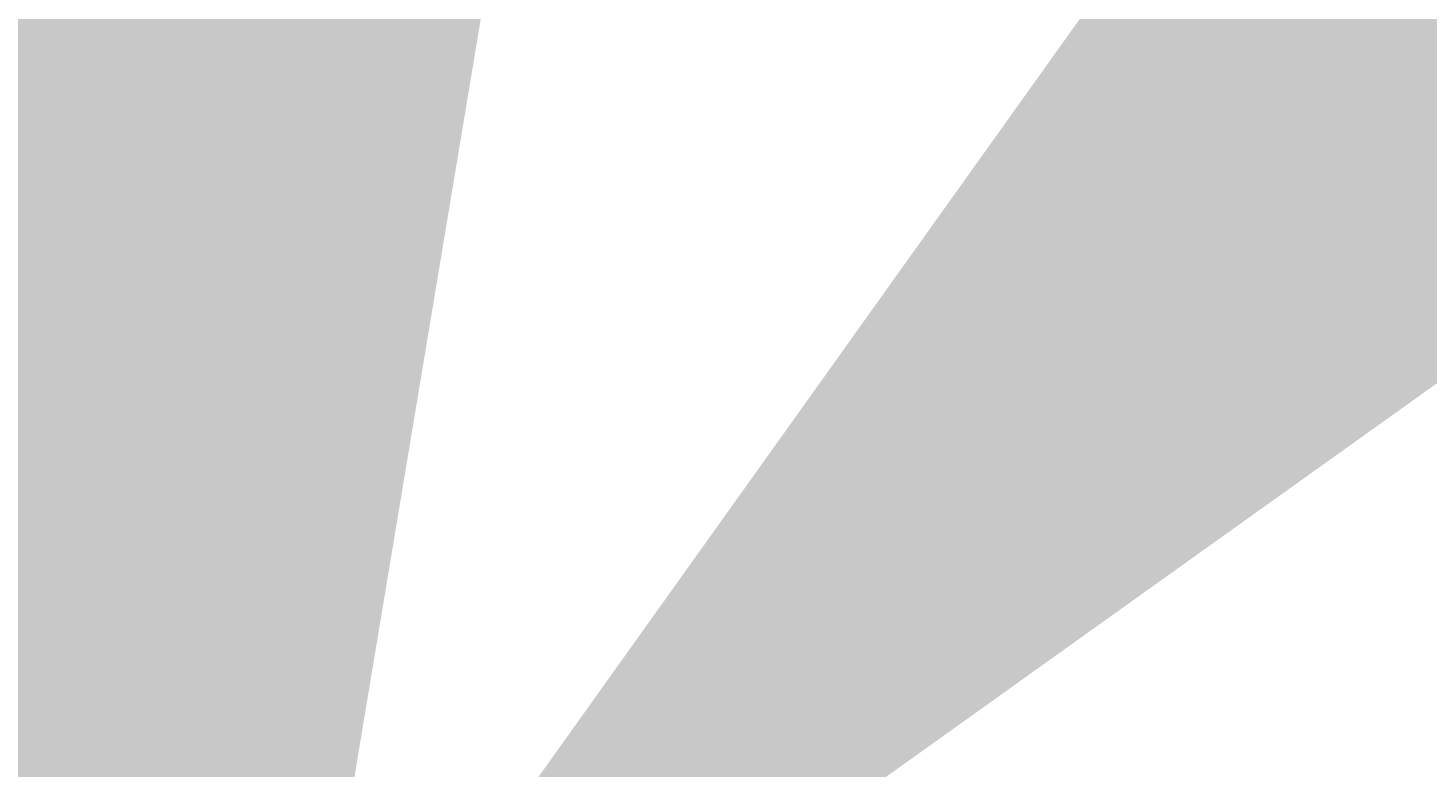
# Model space of a CAD drawing. Units: millimetres. Extents: x -22994 to 29398, y -19990 to 20176.
# Tile 130 of 135: x -44 to 2052, y 895 to 2002. Entities that reach past the tile are written whole.
import ezdxf

# ---------------------------------------------------------------- set-up
doc = ezdxf.new("R2010")
doc.units = ezdxf.units.MM
doc.header["$MEASUREMENT"] = 0
doc.layers.add('M-DIMS', color=2, linetype='Continuous', lineweight=18)
doc.styles.get("Standard").update_dxf_attribs({"font": 'arial.ttf'})
doc.dimstyles.get("Standard").update_dxf_attribs({"dimtxt": 0.18, "dimasz": 10000, "dimexe": 0.18, "dimexo": 0.0625, "dimgap": 0.09, "dimtad": 0, "dimtih": 1, "dimtoh": 1, "dimdec": 0, "dimzin": 0, "dimdsep": 46, "dimtxsty": 'Standard', "dimcen": 0.09, "dimadec": 0, "dimazin": 0, "dimtfac": 1, "dimtdec": 0, "dimtofl": 0, "dimtmove": 0, "dimatfit": 3, "dimfxl": 1, "dimtolj": 1, "dimtzin": 0, "dimlwd": 30, "dimarcsym": 0})

# ---------------------------------------------------------------- blocks, each defined once
blk = doc.blocks.new('*D2')
at = {"layer": 'Defpoints', "color": 0, "transparency": 16777216}
for p in [(6.7, 10.3), (290.9, 10.3), (290.9, -5.1)]:
    blk.add_point(p, dxfattribs=at)
at = {"layer": 'M-DIMS', "color": 0, "lineweight": -2, "transparency": 16777216}
for p, q in [((6.7, 10.2), (6.7, -5.3)), ((290.9, 10.2), (290.9, -5.3))]:
    blk.add_line(p, q, dxfattribs=at)
at = {"layer": 'M-DIMS', "color": 0, "lineweight": 30, "transparency": 16777216}
for p, q in [((-9993.3, -5.1), (-19993.3, -5.1)), ((10290.9, -5.1), (20290.9, -5.1))]:
    blk.add_line(p, q, dxfattribs=at)
at = {"layer": 'M-DIMS', "color": 0, "transparency": 16777216}
for points in [[(-9993.3, 1661.6), (-9993.3, -1671.7), (6.7, -5.1)], [(10290.9, 1661.6), (10290.9, -1671.7), (290.9, -5.1)]]:
    blk.add_solid(points, dxfattribs=at)
at = {"layer": 'M-DIMS', "color": 0, "transparency": 16777216, "insert": (148.8, -5.1), "char_height": 0.18, "attachment_point": 5}
blk.add_mtext('\\A1;284.2', dxfattribs=at)
blk = doc.blocks.new('*D3')
at = {"layer": 'Defpoints', "color": 0, "transparency": 16777216}
for p in [(110.3, 204.2), (110.3, 176.4), (95.8, 128)]:
    blk.add_point(p, dxfattribs=at)
at = {"layer": 'M-DIMS', "color": 0, "lineweight": 30, "transparency": 16777216}
for p, q in [((-9904.2, 204.2), (-19904.2, 204.2)), ((10110.3, 204.2), (20110.3, 204.2))]:
    blk.add_line(p, q, dxfattribs=at)
at = {"layer": 'M-DIMS', "color": 0, "lineweight": -2, "transparency": 16777216}
for p, q in [((95.8, 128), (95.8, 204.3)), ((110.3, 176.4), (110.3, 204.3))]:
    blk.add_line(p, q, dxfattribs=at)
at = {"layer": 'M-DIMS', "color": 0, "transparency": 16777216}
for points in [[(-9904.2, 1870.8), (-9904.2, -1462.5), (95.8, 204.2)], [(10110.3, 1870.8), (10110.3, -1462.5), (110.3, 204.2)]]:
    blk.add_solid(points, dxfattribs=at)
at = {"layer": 'M-DIMS', "color": 0, "transparency": 16777216, "insert": (103, 204.2), "char_height": 0.18, "attachment_point": 5}
blk.add_mtext('\\A1;14.432', dxfattribs=at)
blk = doc.blocks.new('*D4')
at = {"layer": 'Defpoints', "color": 0, "transparency": 16777216}
for p in [(116.3, 204.2), (110.3, 176.4), (116.3, 176.4)]:
    blk.add_point(p, dxfattribs=at)
at = {"layer": 'M-DIMS', "color": 0, "lineweight": 30, "transparency": 16777216}
for p, q in [((-9889.7, 204.2), (-19889.7, 204.2)), ((10116.3, 204.2), (20116.3, 204.2))]:
    blk.add_line(p, q, dxfattribs=at)
at = {"layer": 'M-DIMS', "color": 0, "lineweight": -2, "transparency": 16777216}
for p, q in [((110.3, 176.4), (110.3, 204.3)), ((116.3, 176.4), (116.3, 204.3))]:
    blk.add_line(p, q, dxfattribs=at)
at = {"layer": 'M-DIMS', "color": 0, "transparency": 16777216}
for points in [[(-9889.7, 1870.8), (-9889.7, -1462.5), (110.3, 204.2)], [(10116.3, 1870.8), (10116.3, -1462.5), (116.3, 204.2)]]:
    blk.add_solid(points, dxfattribs=at)
at = {"layer": 'M-DIMS', "color": 0, "transparency": 16777216, "insert": (113.3, 204.2), "char_height": 0.18, "attachment_point": 5}
blk.add_mtext('\\A1;6', dxfattribs=at)
blk = doc.blocks.new('*D5')
at = {"layer": 'Defpoints', "color": 0, "transparency": 16777216}
for p in [(181.3, 204.2), (116.3, 176.4), (181.3, 176.4)]:
    blk.add_point(p, dxfattribs=at)
at = {"layer": 'M-DIMS', "color": 0, "lineweight": 30, "transparency": 16777216}
for p, q in [((-9883.7, 204.2), (-19883.7, 204.2)), ((10181.3, 204.2), (20181.3, 204.2))]:
    blk.add_line(p, q, dxfattribs=at)
at = {"layer": 'M-DIMS', "color": 0, "lineweight": -2, "transparency": 16777216}
for p, q in [((116.3, 176.4), (116.3, 204.3)), ((181.3, 176.4), (181.3, 204.3))]:
    blk.add_line(p, q, dxfattribs=at)
at = {"layer": 'M-DIMS', "color": 0, "transparency": 16777216}
for points in [[(-9883.7, 1870.8), (-9883.7, -1462.5), (116.3, 204.2)], [(10181.3, 1870.8), (10181.3, -1462.5), (181.3, 204.2)]]:
    blk.add_solid(points, dxfattribs=at)
at = {"layer": 'M-DIMS', "color": 0, "transparency": 16777216, "insert": (148.8, 204.2), "char_height": 0.18, "attachment_point": 5}
blk.add_mtext('\\A1;65', dxfattribs=at)
blk = doc.blocks.new('*D6')
at = {"layer": 'Defpoints', "color": 0, "transparency": 16777216}
for p in [(187.3, 204.2), (181.3, 176.4), (187.3, 176.4)]:
    blk.add_point(p, dxfattribs=at)
at = {"layer": 'M-DIMS', "color": 0, "lineweight": 30, "transparency": 16777216}
for p, q in [((-9818.7, 204.2), (-19818.7, 204.2)), ((10187.3, 204.2), (20187.3, 204.2))]:
    blk.add_line(p, q, dxfattribs=at)
at = {"layer": 'M-DIMS', "color": 0, "lineweight": -2, "transparency": 16777216}
for p, q in [((181.3, 176.4), (181.3, 204.3)), ((187.3, 176.4), (187.3, 204.3))]:
    blk.add_line(p, q, dxfattribs=at)
at = {"layer": 'M-DIMS', "color": 0, "transparency": 16777216}
for points in [[(-9818.7, 1870.8), (-9818.7, -1462.5), (181.3, 204.2)], [(10187.3, 1870.8), (10187.3, -1462.5), (187.3, 204.2)]]:
    blk.add_solid(points, dxfattribs=at)
at = {"layer": 'M-DIMS', "color": 0, "transparency": 16777216, "insert": (184.3, 204.2), "char_height": 0.18, "attachment_point": 5}
blk.add_mtext('\\A1;6', dxfattribs=at)
blk = doc.blocks.new('*D7')
at = {"layer": 'Defpoints', "color": 0, "transparency": 16777216}
for p in [(201.7, 204.2), (187.3, 176.4), (201.7, 128)]:
    blk.add_point(p, dxfattribs=at)
at = {"layer": 'M-DIMS', "color": 0, "lineweight": 30, "transparency": 16777216}
for p, q in [((-9812.7, 204.2), (-19812.7, 204.2)), ((10201.7, 204.2), (20201.7, 204.2))]:
    blk.add_line(p, q, dxfattribs=at)
at = {"layer": 'M-DIMS', "color": 0, "lineweight": -2, "transparency": 16777216}
for p, q in [((187.3, 176.4), (187.3, 204.3)), ((201.7, 128), (201.7, 204.3))]:
    blk.add_line(p, q, dxfattribs=at)
at = {"layer": 'M-DIMS', "color": 0, "transparency": 16777216}
for points in [[(-9812.7, 1870.8), (-9812.7, -1462.5), (187.3, 204.2)], [(10201.7, 1870.8), (10201.7, -1462.5), (201.7, 204.2)]]:
    blk.add_solid(points, dxfattribs=at)
at = {"layer": 'M-DIMS', "color": 0, "transparency": 16777216, "insert": (194.5, 204.2), "char_height": 0.18, "attachment_point": 5}
blk.add_mtext('\\A1;14.432', dxfattribs=at)
blk = doc.blocks.new('*D8')
at = {"layer": 'Defpoints', "color": 0, "transparency": 16777216}
for p in [(227.6, 204.2), (227.6, 146.7), (201.7, 128)]:
    blk.add_point(p, dxfattribs=at)
at = {"layer": 'M-DIMS', "color": 0, "lineweight": 30, "transparency": 16777216}
for p, q in [((-9798.3, 204.2), (-19798.3, 204.2)), ((10227.6, 204.2), (20227.6, 204.2))]:
    blk.add_line(p, q, dxfattribs=at)
at = {"layer": 'M-DIMS', "color": 0, "lineweight": -2, "transparency": 16777216}
for p, q in [((201.7, 128), (201.7, 204.3)), ((227.6, 146.8), (227.6, 204.3))]:
    blk.add_line(p, q, dxfattribs=at)
at = {"layer": 'M-DIMS', "color": 0, "transparency": 16777216}
for points in [[(-9798.3, 1870.8), (-9798.3, -1462.5), (201.7, 204.2)], [(10227.6, 1870.8), (10227.6, -1462.5), (227.6, 204.2)]]:
    blk.add_solid(points, dxfattribs=at)
at = {"layer": 'M-DIMS', "color": 0, "transparency": 16777216, "insert": (214.7, 204.2), "char_height": 0.18, "attachment_point": 5}
blk.add_mtext('\\A1;25.95', dxfattribs=at)
blk = doc.blocks.new('*D9')
at = {"layer": 'Defpoints', "color": 0, "transparency": 16777216}
for p in [(187.3, 176.4), (306.2, 176.4), (290.9, 10.3)]:
    blk.add_point(p, dxfattribs=at)
at = {"layer": 'M-DIMS', "color": 0, "lineweight": 30, "transparency": 16777216}
for p, q in [((306.2, 10176.4), (306.2, 20176.4)), ((306.2, -9989.7), (306.2, -19989.7))]:
    blk.add_line(p, q, dxfattribs=at)
at = {"layer": 'M-DIMS', "color": 0, "lineweight": -2, "transparency": 16777216}
for p, q in [((187.3, 176.4), (306.4, 176.4)), ((290.9, 10.3), (306.4, 10.3))]:
    blk.add_line(p, q, dxfattribs=at)
at = {"layer": 'M-DIMS', "color": 0, "transparency": 16777216}
for points in [[(-1360.5, 10176.4), (1972.9, 10176.4), (306.2, 176.4)], [(-1360.5, -9989.7), (1972.9, -9989.7), (306.2, 10.3)]]:
    blk.add_solid(points, dxfattribs=at)
at = {"layer": 'M-DIMS', "color": 0, "transparency": 16777216, "insert": (306.2, 93.3), "char_height": 0.18, "attachment_point": 5}
blk.add_mtext('\\A1;166.1', dxfattribs=at)
blk = doc.blocks.new('*D10')
at = {"layer": 'Defpoints', "color": 0, "transparency": 16777216}
for p in [(125.6, 136.1), (133.3, 136.1), (133.3, -5.1)]:
    blk.add_point(p, dxfattribs=at)
at = {"layer": 'M-DIMS', "color": 0, "lineweight": -2, "transparency": 16777216}
for p, q in [((125.6, 136), (125.6, -5.3)), ((133.3, 136), (133.3, -5.3))]:
    blk.add_line(p, q, dxfattribs=at)
at = {"layer": 'M-DIMS', "color": 0, "lineweight": 30, "transparency": 16777216}
for p, q in [((-9874.4, -5.1), (-19874.4, -5.1)), ((10133.3, -5.1), (20133.3, -5.1))]:
    blk.add_line(p, q, dxfattribs=at)
at = {"layer": 'M-DIMS', "color": 0, "transparency": 16777216}
for points in [[(-9874.4, 1661.6), (-9874.4, -1671.7), (125.6, -5.1)], [(10133.3, 1661.6), (10133.3, -1671.7), (133.3, -5.1)]]:
    blk.add_solid(points, dxfattribs=at)
at = {"layer": 'M-DIMS', "color": 0, "transparency": 16777216, "insert": (129.5, -5.1), "char_height": 0.18, "attachment_point": 5}
blk.add_mtext('\\A1;7.696', dxfattribs=at)
blk = doc.blocks.new('*D11')
at = {"layer": 'Defpoints', "color": 0, "transparency": 16777216}
for p in [(133.3, 136.1), (135.6, 136.1), (135.6, -5.1)]:
    blk.add_point(p, dxfattribs=at)
at = {"layer": 'M-DIMS', "color": 0, "lineweight": -2, "transparency": 16777216}
for p, q in [((133.3, 136), (133.3, -5.3)), ((135.6, 136), (135.6, -5.3))]:
    blk.add_line(p, q, dxfattribs=at)
at = {"layer": 'M-DIMS', "color": 0, "lineweight": 30, "transparency": 16777216}
for p, q in [((-9866.7, -5.1), (-19866.7, -5.1)), ((10135.6, -5.1), (20135.6, -5.1))]:
    blk.add_line(p, q, dxfattribs=at)
at = {"layer": 'M-DIMS', "color": 0, "transparency": 16777216}
for points in [[(-9866.7, 1661.6), (-9866.7, -1671.7), (133.3, -5.1)], [(10135.6, 1661.6), (10135.6, -1671.7), (135.6, -5.1)]]:
    blk.add_solid(points, dxfattribs=at)
at = {"layer": 'M-DIMS', "color": 0, "transparency": 16777216, "insert": (134.5, -5.1), "char_height": 0.18, "attachment_point": 5}
blk.add_mtext('\\A1;2.304', dxfattribs=at)
blk = doc.blocks.new('*D12')
at = {"layer": 'Defpoints', "color": 0, "transparency": 16777216}
for p in [(135.6, 136.1), (145.6, 136.1), (145.6, -5.1)]:
    blk.add_point(p, dxfattribs=at)
at = {"layer": 'M-DIMS', "color": 0, "lineweight": -2, "transparency": 16777216}
for p, q in [((135.6, 136), (135.6, -5.3)), ((145.6, 136), (145.6, -5.3))]:
    blk.add_line(p, q, dxfattribs=at)
at = {"layer": 'M-DIMS', "color": 0, "lineweight": 30, "transparency": 16777216}
for p, q in [((-9864.4, -5.1), (-19864.4, -5.1)), ((10145.6, -5.1), (20145.6, -5.1))]:
    blk.add_line(p, q, dxfattribs=at)
at = {"layer": 'M-DIMS', "color": 0, "transparency": 16777216}
for points in [[(-9864.4, 1661.6), (-9864.4, -1671.7), (135.6, -5.1)], [(10145.6, 1661.6), (10145.6, -1671.7), (145.6, -5.1)]]:
    blk.add_solid(points, dxfattribs=at)
at = {"layer": 'M-DIMS', "color": 0, "transparency": 16777216, "insert": (140.6, -5.1), "char_height": 0.18, "attachment_point": 5}
blk.add_mtext('\\A1;10', dxfattribs=at)
blk = doc.blocks.new('*D13')
at = {"layer": 'Defpoints', "color": 0, "transparency": 16777216}
for p in [(145.6, 136.1), (155.6, 136.1), (155.6, -5.1)]:
    blk.add_point(p, dxfattribs=at)
at = {"layer": 'M-DIMS', "color": 0, "lineweight": -2, "transparency": 16777216}
for p, q in [((145.6, 136), (145.6, -5.3)), ((155.6, 136), (155.6, -5.3))]:
    blk.add_line(p, q, dxfattribs=at)
at = {"layer": 'M-DIMS', "color": 0, "lineweight": 30, "transparency": 16777216}
for p, q in [((-9854.4, -5.1), (-19854.4, -5.1)), ((10155.6, -5.1), (20155.6, -5.1))]:
    blk.add_line(p, q, dxfattribs=at)
at = {"layer": 'M-DIMS', "color": 0, "transparency": 16777216}
for points in [[(-9854.4, 1661.6), (-9854.4, -1671.7), (145.6, -5.1)], [(10155.6, 1661.6), (10155.6, -1671.7), (155.6, -5.1)]]:
    blk.add_solid(points, dxfattribs=at)
at = {"layer": 'M-DIMS', "color": 0, "transparency": 16777216, "insert": (150.6, -5.1), "char_height": 0.18, "attachment_point": 5}
blk.add_mtext('\\A1;10', dxfattribs=at)
blk = doc.blocks.new('*D14')
at = {"layer": 'Defpoints', "color": 0, "transparency": 16777216}
for p in [(155.6, 136.1), (165.6, 136.1), (165.6, -5.1)]:
    blk.add_point(p, dxfattribs=at)
at = {"layer": 'M-DIMS', "color": 0, "lineweight": -2, "transparency": 16777216}
for p, q in [((155.6, 136), (155.6, -5.3)), ((165.6, 136), (165.6, -5.3))]:
    blk.add_line(p, q, dxfattribs=at)
at = {"layer": 'M-DIMS', "color": 0, "lineweight": 30, "transparency": 16777216}
for p, q in [((-9844.4, -5.1), (-19844.4, -5.1)), ((10165.6, -5.1), (20165.6, -5.1))]:
    blk.add_line(p, q, dxfattribs=at)
at = {"layer": 'M-DIMS', "color": 0, "transparency": 16777216}
for points in [[(-9844.4, 1661.6), (-9844.4, -1671.7), (155.6, -5.1)], [(10165.6, 1661.6), (10165.6, -1671.7), (165.6, -5.1)]]:
    blk.add_solid(points, dxfattribs=at)
at = {"layer": 'M-DIMS', "color": 0, "transparency": 16777216, "insert": (160.6, -5.1), "char_height": 0.18, "attachment_point": 5}
blk.add_mtext('\\A1;10', dxfattribs=at)
blk = doc.blocks.new('*D15')
at = {"layer": 'Defpoints', "color": 0, "transparency": 16777216}
for p in [(173.3, 154.8), (173.3, 136.1), (306.2, 136.1)]:
    blk.add_point(p, dxfattribs=at)
at = {"layer": 'M-DIMS', "color": 0, "lineweight": 30, "transparency": 16777216}
for p, q in [((306.2, 10154.8), (306.2, 20154.8)), ((306.2, -9863.9), (306.2, -19863.9))]:
    blk.add_line(p, q, dxfattribs=at)
at = {"layer": 'M-DIMS', "color": 0, "lineweight": -2, "transparency": 16777216}
for p, q in [((173.4, 154.8), (306.4, 154.8)), ((173.4, 136.1), (306.4, 136.1))]:
    blk.add_line(p, q, dxfattribs=at)
at = {"layer": 'M-DIMS', "color": 0, "transparency": 16777216}
for points in [[(-1360.5, 10154.8), (1972.9, 10154.8), (306.2, 154.8)], [(-1360.5, -9863.9), (1972.9, -9863.9), (306.2, 136.1)]]:
    blk.add_solid(points, dxfattribs=at)
at = {"layer": 'M-DIMS', "color": 0, "transparency": 16777216, "insert": (306.2, 145.4), "char_height": 0.18, "attachment_point": 5}
blk.add_mtext('\\A1;18.717', dxfattribs=at)
blk = doc.blocks.new('*D16')
at = {"layer": 'Defpoints', "color": 0, "transparency": 16777216}
for p in [(120.2, 204.2), (110.5, 48), (120.2, 48)]:
    blk.add_point(p, dxfattribs=at)
at = {"layer": 'M-DIMS', "color": 0, "lineweight": 30, "transparency": 16777216}
for p, q in [((-9889.5, 204.2), (-19889.5, 204.2)), ((10120.2, 204.2), (20120.2, 204.2))]:
    blk.add_line(p, q, dxfattribs=at)
at = {"layer": 'M-DIMS', "color": 0, "lineweight": -2, "transparency": 16777216}
for p, q in [((110.5, 48.1), (110.5, 204.3)), ((120.2, 48.1), (120.2, 204.3))]:
    blk.add_line(p, q, dxfattribs=at)
at = {"layer": 'M-DIMS', "color": 0, "transparency": 16777216}
for points in [[(-9889.5, 1870.8), (-9889.5, -1462.5), (110.5, 204.2)], [(10120.2, 1870.8), (10120.2, -1462.5), (120.2, 204.2)]]:
    blk.add_solid(points, dxfattribs=at)
at = {"layer": 'M-DIMS', "color": 0, "transparency": 16777216, "insert": (115.3, 204.2), "char_height": 0.18, "attachment_point": 5}
blk.add_mtext('\\A1;9.704', dxfattribs=at)
blk = doc.blocks.new('*D17')
at = {"layer": 'Defpoints', "color": 0, "transparency": 16777216}
for p in [(126.2, 204.2), (120.2, 48), (126.2, 48)]:
    blk.add_point(p, dxfattribs=at)
at = {"layer": 'M-DIMS', "color": 0, "lineweight": 30, "transparency": 16777216}
for p, q in [((-9879.8, 204.2), (-19879.8, 204.2)), ((10126.2, 204.2), (20126.2, 204.2))]:
    blk.add_line(p, q, dxfattribs=at)
at = {"layer": 'M-DIMS', "color": 0, "lineweight": -2, "transparency": 16777216}
for p, q in [((120.2, 48.1), (120.2, 204.3)), ((126.2, 48.1), (126.2, 204.3))]:
    blk.add_line(p, q, dxfattribs=at)
at = {"layer": 'M-DIMS', "color": 0, "transparency": 16777216}
for points in [[(-9879.8, 1870.8), (-9879.8, -1462.5), (120.2, 204.2)], [(10126.2, 1870.8), (10126.2, -1462.5), (126.2, 204.2)]]:
    blk.add_solid(points, dxfattribs=at)
at = {"layer": 'M-DIMS', "color": 0, "transparency": 16777216, "insert": (123.2, 204.2), "char_height": 0.18, "attachment_point": 5}
blk.add_mtext('\\A1;6', dxfattribs=at)
blk = doc.blocks.new('*D18')
at = {"layer": 'Defpoints', "color": 0, "transparency": 16777216}
for p in [(132.2, 204.2), (126.2, 48), (132.2, 48)]:
    blk.add_point(p, dxfattribs=at)
at = {"layer": 'M-DIMS', "color": 0, "lineweight": 30, "transparency": 16777216}
for p, q in [((-9873.8, 204.2), (-19873.8, 204.2)), ((10132.2, 204.2), (20132.2, 204.2))]:
    blk.add_line(p, q, dxfattribs=at)
at = {"layer": 'M-DIMS', "color": 0, "lineweight": -2, "transparency": 16777216}
for p, q in [((126.2, 48.1), (126.2, 204.3)), ((132.2, 48.1), (132.2, 204.3))]:
    blk.add_line(p, q, dxfattribs=at)
at = {"layer": 'M-DIMS', "color": 0, "transparency": 16777216}
for points in [[(-9873.8, 1870.8), (-9873.8, -1462.5), (126.2, 204.2)], [(10132.2, 1870.8), (10132.2, -1462.5), (132.2, 204.2)]]:
    blk.add_solid(points, dxfattribs=at)
at = {"layer": 'M-DIMS', "color": 0, "transparency": 16777216, "insert": (129.2, 204.2), "char_height": 0.18, "attachment_point": 5}
blk.add_mtext('\\A1;6', dxfattribs=at)
blk = doc.blocks.new('*D19')
at = {"layer": 'Defpoints', "color": 0, "transparency": 16777216}
for p in [(138.2, 204.2), (132.2, 48), (138.2, 48)]:
    blk.add_point(p, dxfattribs=at)
at = {"layer": 'M-DIMS', "color": 0, "lineweight": 30, "transparency": 16777216}
for p, q in [((-9867.8, 204.2), (-19867.8, 204.2)), ((10138.2, 204.2), (20138.2, 204.2))]:
    blk.add_line(p, q, dxfattribs=at)
at = {"layer": 'M-DIMS', "color": 0, "lineweight": -2, "transparency": 16777216}
for p, q in [((132.2, 48.1), (132.2, 204.3)), ((138.2, 48.1), (138.2, 204.3))]:
    blk.add_line(p, q, dxfattribs=at)
at = {"layer": 'M-DIMS', "color": 0, "transparency": 16777216}
for points in [[(-9867.8, 1870.8), (-9867.8, -1462.5), (132.2, 204.2)], [(10138.2, 1870.8), (10138.2, -1462.5), (138.2, 204.2)]]:
    blk.add_solid(points, dxfattribs=at)
at = {"layer": 'M-DIMS', "color": 0, "transparency": 16777216, "insert": (135.2, 204.2), "char_height": 0.18, "attachment_point": 5}
blk.add_mtext('\\A1;6', dxfattribs=at)
blk = doc.blocks.new('*D20')
at = {"layer": 'Defpoints', "color": 0, "transparency": 16777216}
for p in [(144.2, 204.2), (138.2, 48), (144.2, 48)]:
    blk.add_point(p, dxfattribs=at)
at = {"layer": 'M-DIMS', "color": 0, "lineweight": 30, "transparency": 16777216}
for p, q in [((-9861.8, 204.2), (-19861.8, 204.2)), ((10144.2, 204.2), (20144.2, 204.2))]:
    blk.add_line(p, q, dxfattribs=at)
at = {"layer": 'M-DIMS', "color": 0, "lineweight": -2, "transparency": 16777216}
for p, q in [((138.2, 48.1), (138.2, 204.3)), ((144.2, 48.1), (144.2, 204.3))]:
    blk.add_line(p, q, dxfattribs=at)
at = {"layer": 'M-DIMS', "color": 0, "transparency": 16777216}
for points in [[(-9861.8, 1870.8), (-9861.8, -1462.5), (138.2, 204.2)], [(10144.2, 1870.8), (10144.2, -1462.5), (144.2, 204.2)]]:
    blk.add_solid(points, dxfattribs=at)
at = {"layer": 'M-DIMS', "color": 0, "transparency": 16777216, "insert": (141.2, 204.2), "char_height": 0.18, "attachment_point": 5}
blk.add_mtext('\\A1;6', dxfattribs=at)
blk = doc.blocks.new('*D21')
at = {"layer": 'Defpoints', "color": 0, "transparency": 16777216}
for p in [(149.1, 204.2), (144.2, 48), (149.1, 48)]:
    blk.add_point(p, dxfattribs=at)
at = {"layer": 'M-DIMS', "color": 0, "lineweight": 30, "transparency": 16777216}
for p, q in [((-9855.8, 204.2), (-19855.8, 204.2)), ((10149.1, 204.2), (20149.1, 204.2))]:
    blk.add_line(p, q, dxfattribs=at)
at = {"layer": 'M-DIMS', "color": 0, "lineweight": -2, "transparency": 16777216}
for p, q in [((144.2, 48.1), (144.2, 204.3)), ((149.1, 48.1), (149.1, 204.3))]:
    blk.add_line(p, q, dxfattribs=at)
at = {"layer": 'M-DIMS', "color": 0, "transparency": 16777216}
for points in [[(-9855.8, 1870.8), (-9855.8, -1462.5), (144.2, 204.2)], [(10149.1, 1870.8), (10149.1, -1462.5), (149.1, 204.2)]]:
    blk.add_solid(points, dxfattribs=at)
at = {"layer": 'M-DIMS', "color": 0, "transparency": 16777216, "insert": (146.6, 204.2), "char_height": 0.18, "attachment_point": 5}
blk.add_mtext('\\A1;4.945', dxfattribs=at)
blk = doc.blocks.new('*D22')
at = {"layer": 'Defpoints', "color": 0, "transparency": 16777216}
for p in [(149.1, 31), (155.1, 31), (155.1, -5.1)]:
    blk.add_point(p, dxfattribs=at)
at = {"layer": 'M-DIMS', "color": 0, "lineweight": -2, "transparency": 16777216}
for p, q in [((149.1, 30.9), (149.1, -5.3)), ((155.1, 30.9), (155.1, -5.3))]:
    blk.add_line(p, q, dxfattribs=at)
at = {"layer": 'M-DIMS', "color": 0, "lineweight": 30, "transparency": 16777216}
for p, q in [((-9850.9, -5.1), (-19850.9, -5.1)), ((10155.1, -5.1), (20155.1, -5.1))]:
    blk.add_line(p, q, dxfattribs=at)
at = {"layer": 'M-DIMS', "color": 0, "transparency": 16777216}
for points in [[(-9850.9, 1661.6), (-9850.9, -1671.7), (149.1, -5.1)], [(10155.1, 1661.6), (10155.1, -1671.7), (155.1, -5.1)]]:
    blk.add_solid(points, dxfattribs=at)
at = {"layer": 'M-DIMS', "color": 0, "transparency": 16777216, "insert": (152.1, -5.1), "char_height": 0.18, "attachment_point": 5}
blk.add_mtext('\\A1;6', dxfattribs=at)
blk = doc.blocks.new('*D23')
at = {"layer": 'Defpoints', "color": 0, "transparency": 16777216}
for p in [(155.1, 31), (161.1, 31), (161.1, -5.1)]:
    blk.add_point(p, dxfattribs=at)
at = {"layer": 'M-DIMS', "color": 0, "lineweight": -2, "transparency": 16777216}
for p, q in [((155.1, 30.9), (155.1, -5.3)), ((161.1, 30.9), (161.1, -5.3))]:
    blk.add_line(p, q, dxfattribs=at)
at = {"layer": 'M-DIMS', "color": 0, "lineweight": 30, "transparency": 16777216}
for p, q in [((-9844.9, -5.1), (-19844.9, -5.1)), ((10161.1, -5.1), (20161.1, -5.1))]:
    blk.add_line(p, q, dxfattribs=at)
at = {"layer": 'M-DIMS', "color": 0, "transparency": 16777216}
for points in [[(-9844.9, 1661.6), (-9844.9, -1671.7), (155.1, -5.1)], [(10161.1, 1661.6), (10161.1, -1671.7), (161.1, -5.1)]]:
    blk.add_solid(points, dxfattribs=at)
at = {"layer": 'M-DIMS', "color": 0, "transparency": 16777216, "insert": (158.1, -5.1), "char_height": 0.18, "attachment_point": 5}
blk.add_mtext('\\A1;6', dxfattribs=at)
blk = doc.blocks.new('*D24')
at = {"layer": 'Defpoints', "color": 0, "transparency": 16777216}
for p in [(161.1, 31), (166.4, 31), (166.4, -5.1)]:
    blk.add_point(p, dxfattribs=at)
at = {"layer": 'M-DIMS', "color": 0, "lineweight": -2, "transparency": 16777216}
for p, q in [((161.1, 30.9), (161.1, -5.3)), ((166.4, 30.9), (166.4, -5.3))]:
    blk.add_line(p, q, dxfattribs=at)
at = {"layer": 'M-DIMS', "color": 0, "lineweight": 30, "transparency": 16777216}
for p, q in [((-9838.9, -5.1), (-19838.9, -5.1)), ((10166.4, -5.1), (20166.4, -5.1))]:
    blk.add_line(p, q, dxfattribs=at)
at = {"layer": 'M-DIMS', "color": 0, "transparency": 16777216}
for points in [[(-9838.9, 1661.6), (-9838.9, -1671.7), (161.1, -5.1)], [(10166.4, 1661.6), (10166.4, -1671.7), (166.4, -5.1)]]:
    blk.add_solid(points, dxfattribs=at)
at = {"layer": 'M-DIMS', "color": 0, "transparency": 16777216, "insert": (163.8, -5.1), "char_height": 0.18, "attachment_point": 5}
blk.add_mtext('\\A1;5.323', dxfattribs=at)
blk = doc.blocks.new('*D25')
at = {"layer": 'Defpoints', "color": 0, "transparency": 16777216}
for p in [(166.4, 31), (172.4, 31), (172.4, -5.1)]:
    blk.add_point(p, dxfattribs=at)
at = {"layer": 'M-DIMS', "color": 0, "lineweight": -2, "transparency": 16777216}
for p, q in [((166.4, 30.9), (166.4, -5.3)), ((172.4, 30.9), (172.4, -5.3))]:
    blk.add_line(p, q, dxfattribs=at)
at = {"layer": 'M-DIMS', "color": 0, "lineweight": 30, "transparency": 16777216}
for p, q in [((-9833.6, -5.1), (-19833.6, -5.1)), ((10172.4, -5.1), (20172.4, -5.1))]:
    blk.add_line(p, q, dxfattribs=at)
at = {"layer": 'M-DIMS', "color": 0, "transparency": 16777216}
for points in [[(-9833.6, 1661.6), (-9833.6, -1671.7), (166.4, -5.1)], [(10172.4, 1661.6), (10172.4, -1671.7), (172.4, -5.1)]]:
    blk.add_solid(points, dxfattribs=at)
at = {"layer": 'M-DIMS', "color": 0, "transparency": 16777216, "insert": (169.4, -5.1), "char_height": 0.18, "attachment_point": 5}
blk.add_mtext('\\A1;6', dxfattribs=at)
blk = doc.blocks.new('*D26')
at = {"layer": 'Defpoints', "color": 0, "transparency": 16777216}
for p in [(172.4, 31), (178.4, 31), (178.4, -5.1)]:
    blk.add_point(p, dxfattribs=at)
at = {"layer": 'M-DIMS', "color": 0, "lineweight": -2, "transparency": 16777216}
for p, q in [((172.4, 30.9), (172.4, -5.3)), ((178.4, 30.9), (178.4, -5.3))]:
    blk.add_line(p, q, dxfattribs=at)
at = {"layer": 'M-DIMS', "color": 0, "lineweight": 30, "transparency": 16777216}
for p, q in [((-9827.6, -5.1), (-19827.6, -5.1)), ((10178.4, -5.1), (20178.4, -5.1))]:
    blk.add_line(p, q, dxfattribs=at)
at = {"layer": 'M-DIMS', "color": 0, "transparency": 16777216}
for points in [[(-9827.6, 1661.6), (-9827.6, -1671.7), (172.4, -5.1)], [(10178.4, 1661.6), (10178.4, -1671.7), (178.4, -5.1)]]:
    blk.add_solid(points, dxfattribs=at)
at = {"layer": 'M-DIMS', "color": 0, "transparency": 16777216, "insert": (175.4, -5.1), "char_height": 0.18, "attachment_point": 5}
blk.add_mtext('\\A1;6', dxfattribs=at)
blk = doc.blocks.new('*D27')
at = {"layer": 'Defpoints', "color": 0, "transparency": 16777216}
for p in [(178.4, 31), (188.1, 31), (188.1, -5.1)]:
    blk.add_point(p, dxfattribs=at)
at = {"layer": 'M-DIMS', "color": 0, "lineweight": -2, "transparency": 16777216}
for p, q in [((178.4, 30.9), (178.4, -5.3)), ((188.1, 30.9), (188.1, -5.3))]:
    blk.add_line(p, q, dxfattribs=at)
at = {"layer": 'M-DIMS', "color": 0, "lineweight": 30, "transparency": 16777216}
for p, q in [((-9821.6, -5.1), (-19821.6, -5.1)), ((10188.1, -5.1), (20188.1, -5.1))]:
    blk.add_line(p, q, dxfattribs=at)
at = {"layer": 'M-DIMS', "color": 0, "transparency": 16777216}
for points in [[(-9821.6, 1661.6), (-9821.6, -1671.7), (178.4, -5.1)], [(10188.1, 1661.6), (10188.1, -1671.7), (188.1, -5.1)]]:
    blk.add_solid(points, dxfattribs=at)
at = {"layer": 'M-DIMS', "color": 0, "transparency": 16777216, "insert": (183.3, -5.1), "char_height": 0.18, "attachment_point": 5}
blk.add_mtext('\\A1;9.679', dxfattribs=at)
blk = doc.blocks.new('*D28')
at = {"layer": 'Defpoints', "color": 0, "transparency": 16777216}
for p in [(188.1, 48), (306.2, 48), (188.1, 31)]:
    blk.add_point(p, dxfattribs=at)
at = {"layer": 'M-DIMS', "color": 0, "lineweight": 30, "transparency": 16777216}
for p, q in [((306.2, 10048), (306.2, 20048)), ((306.2, -9969), (306.2, -19969))]:
    blk.add_line(p, q, dxfattribs=at)
at = {"layer": 'M-DIMS', "color": 0, "lineweight": -2, "transparency": 16777216}
for p, q in [((188.2, 48), (306.4, 48)), ((188.2, 31), (306.4, 31))]:
    blk.add_line(p, q, dxfattribs=at)
at = {"layer": 'M-DIMS', "color": 0, "transparency": 16777216}
for points in [[(-1360.5, 10048), (1972.9, 10048), (306.2, 48)], [(-1360.5, -9969), (1972.9, -9969), (306.2, 31)]]:
    blk.add_solid(points, dxfattribs=at)
at = {"layer": 'M-DIMS', "color": 0, "transparency": 16777216, "insert": (306.2, 39.5), "char_height": 0.18, "attachment_point": 5}
blk.add_mtext('\\A1;17.045', dxfattribs=at)
blk = doc.blocks.new('*D29')
at = {"layer": 'Defpoints', "color": 0, "transparency": 16777216}
for p in [(36.8, 80), (64, 80)]:
    blk.add_point(p, dxfattribs=at)
at = {"layer": 'M-DIMS', "color": 0, "lineweight": -2, "transparency": 16777216}
for p, q in [((50.3, 80), (50.5, 80)), ((50.4, 80), (50.4, 80.1))]:
    blk.add_line(p, q, dxfattribs=at)
at = {"layer": 'M-DIMS', "color": 0, "lineweight": 30, "transparency": 16777216}
blk.add_line((20064, 80), (10064, 80), dxfattribs=at)
at = {"layer": 'M-DIMS', "color": 0, "transparency": 16777216}
blk.add_solid([(10064, 1746.7), (10064, -1586.6), (64, 80)], dxfattribs=at)
at = {"layer": 'M-DIMS', "color": 0, "transparency": 16777216, "insert": (20064.5, 80), "char_height": 0.18, "attachment_point": 5}
blk.add_mtext('\\A1;∅27.23', dxfattribs=at)
blk = doc.blocks.new('*D30')
at = {"layer": 'Defpoints', "color": 0, "transparency": 16777216}
for p in [(216.3, 146.7), (239, 146.7)]:
    blk.add_point(p, dxfattribs=at)
at = {"layer": 'M-DIMS', "color": 0, "lineweight": -2, "transparency": 16777216}
for p, q in [((227.6, 146.6), (227.6, 146.8)), ((227.6, 146.7), (227.7, 146.7))]:
    blk.add_line(p, q, dxfattribs=at)
at = {"layer": 'M-DIMS', "color": 0, "lineweight": 30, "transparency": 16777216}
blk.add_line((20239, 147.5), (10239, 147.1), dxfattribs=at)
at = {"layer": 'M-DIMS', "color": 0, "transparency": 16777216}
blk.add_solid([(10238.9, 1813.8), (10239, -1519.6), (239, 146.7)], dxfattribs=at)
at = {"layer": 'M-DIMS', "color": 0, "transparency": 16777216, "insert": (20239.5, 147.5), "char_height": 0.18, "attachment_point": 5}
blk.add_mtext('\\A1;∅22.667', dxfattribs=at)
blk = doc.blocks.new('*D31')
at = {"layer": 'Defpoints', "color": 0, "transparency": 16777216}
for p in [(223.2, 146.7), (232.1, 146.7)]:
    blk.add_point(p, dxfattribs=at)
at = {"layer": 'M-DIMS', "color": 0, "lineweight": -2, "transparency": 16777216}
for p, q in [((227.6, 146.6), (227.6, 146.8)), ((227.6, 146.7), (227.7, 146.7))]:
    blk.add_line(p, q, dxfattribs=at)
at = {"layer": 'M-DIMS', "color": 0, "lineweight": 30, "transparency": 16777216}
blk.add_line((20232.1, 148.7), (10232.1, 147.7), dxfattribs=at)
at = {"layer": 'M-DIMS', "color": 0, "transparency": 16777216}
blk.add_solid([(10232, 1814.4), (10232.3, -1519), (232.1, 146.7)], dxfattribs=at)
at = {"layer": 'M-DIMS', "color": 0, "transparency": 16777216, "insert": (20232.6, 148.7), "char_height": 0.18, "attachment_point": 5}
blk.add_mtext('\\A1;∅8.969', dxfattribs=at)
blk = doc.blocks.new('*D34')
at = {"layer": 'Defpoints', "color": 0, "transparency": 16777216}
for p in [(176.8, 121.1), (178.6, 122.9)]:
    blk.add_point(p, dxfattribs=at)
at = {"layer": 'M-DIMS', "color": 0, "lineweight": 30, "transparency": 16777216}
for p, q in [((14322.4, 14263.3), (7250.5, 7193.1)), ((24322.4, 14263.3), (14322.4, 14263.3))]:
    blk.add_line(p, q, dxfattribs=at)
at = {"layer": 'M-DIMS', "color": 0, "lineweight": -2, "transparency": 16777216}
for p, q in [((176.7, 121.1), (176.9, 121.1)), ((176.8, 121), (176.8, 121.2))]:
    blk.add_line(p, q, dxfattribs=at)
at = {"layer": 'M-DIMS', "color": 0, "transparency": 16777216}
blk.add_solid([(6072.1, 8371.8), (8428.9, 6014.4), (178.6, 122.9)], dxfattribs=at)
at = {"layer": 'M-DIMS', "color": 0, "transparency": 16777216, "insert": (24323, 14263.3), "char_height": 0.18, "attachment_point": 5}
blk.add_mtext('\\A1;6X R2.5', dxfattribs=at)
blk = doc.blocks.new('*D35')
at = {"layer": 'Defpoints', "color": 0, "transparency": 16777216}
for p in [(21.1, 77.4), (21.8, 76.1)]:
    blk.add_point(p, dxfattribs=at)
at = {"layer": 'M-DIMS', "color": 0, "lineweight": 30, "transparency": 16777216}
for p, q in [((-19938, 17421.4), (-9938, 17421.4)), ((-9938, 17421.4), (-4958.5, 8749.4))]:
    blk.add_line(p, q, dxfattribs=at)
at = {"layer": 'M-DIMS', "color": 0, "lineweight": -2, "transparency": 16777216}
for p, q in [((21.8, 76), (21.8, 76.2)), ((21.8, 76.1), (21.9, 76.1))]:
    blk.add_line(p, q, dxfattribs=at)
at = {"layer": 'M-DIMS', "color": 0, "transparency": 16777216}
blk.add_solid([(-3513.1, 9579.3), (-6403.8, 7919.5), (21.1, 77.4)], dxfattribs=at)
at = {"layer": 'M-DIMS', "color": 0, "transparency": 16777216, "insert": (-19938.4, 17421.4), "char_height": 0.18, "attachment_point": 5}
blk.add_mtext('\\A1;R1.5', dxfattribs=at)
blk = doc.blocks.new('*D36')
at = {"layer": 'Defpoints', "color": 0, "transparency": 16777216}
for p in [(46.4, 31.3), (46.4, 26.6)]:
    blk.add_point(p, dxfattribs=at)
at = {"layer": 'M-DIMS', "color": 0, "lineweight": 30, "transparency": 16777216}
for p, q in [((57.1, 20031.3), (51.8, 10031.3)), ((10057.1, 20031.3), (57.1, 20031.3))]:
    blk.add_line(p, q, dxfattribs=at)
at = {"layer": 'M-DIMS', "color": 0, "lineweight": -2, "transparency": 16777216}
for p, q in [((46.3, 28.9), (46.5, 28.9)), ((46.4, 28.9), (46.4, 29))]:
    blk.add_line(p, q, dxfattribs=at)
at = {"layer": 'M-DIMS', "color": 0, "transparency": 16777216}
blk.add_solid([(-1614.9, 10032.2), (1718.4, 10030.4), (46.4, 31.3)], dxfattribs=at)
at = {"layer": 'M-DIMS', "color": 0, "transparency": 16777216, "insert": (10057.6, 20031.3), "char_height": 0.18, "attachment_point": 5}
blk.add_mtext('\\A1;∅4.71', dxfattribs=at)
blk = doc.blocks.new('*D37')
at = {"layer": 'Defpoints', "color": 0, "transparency": 16777216}
for p in [(54.8, 118.6), (59.5, 118.6)]:
    blk.add_point(p, dxfattribs=at)
at = {"layer": 'M-DIMS', "color": 0, "lineweight": -2, "transparency": 16777216}
for p, q in [((57.1, 118.6), (57.3, 118.6)), ((57.2, 118.5), (57.2, 118.7))]:
    blk.add_line(p, q, dxfattribs=at)
at = {"layer": 'M-DIMS', "color": 0, "lineweight": 30, "transparency": 16777216}
blk.add_line((20059.5, 116.3), (10059.5, 117.4), dxfattribs=at)
at = {"layer": 'M-DIMS', "color": 0, "transparency": 16777216}
blk.add_solid([(10059.7, 1784.1), (10059.3, -1549.2), (59.5, 118.6)], dxfattribs=at)
at = {"layer": 'M-DIMS', "color": 0, "transparency": 16777216, "insert": (20060, 116.3), "char_height": 0.18, "attachment_point": 5}
blk.add_mtext('\\A1;∅4.659', dxfattribs=at)

msp = doc.modelspace()

# ---------------------------------------------------------------- dimensions: what is measured, and where the dimension line sits
at = {"layer": 'M-DIMS'}
for base, p1, p2, override, picture, middle in [((306.202, 176.3662), (290.852, 10.2713), (187.2647, 176.3662), {"dimdec": 1, "dimlfac": 1, "dimrnd": 0, "dimzin": 0, "dimdsep": 46, "dimlunit": 2}, '*D9', (306.202, 93.3187)), ((306.202, 136.0713), (173.3459, 154.788), (173.3459, 136.0713), {"dimdec": 3, "dimlfac": 1, "dimrnd": 0, "dimzin": 0, "dimdsep": 46, "dimlunit": 2}, '*D15', (306.202, 145.4297)), ((306.202, 48.0349), (188.1175, 30.9895), (188.1175, 48.0349), {"dimdec": 3, "dimlfac": 1, "dimrnd": 0, "dimzin": 0, "dimdsep": 46, "dimlunit": 2}, '*D28', (306.202, 39.5122))]:
    dim = msp.add_linear_dim(base=base, p1=p1, p2=p2, angle=90, dimstyle='Standard', override=override, dxfattribs=at)
    dim.commit()
    dim.dimension.update_dxf_attribs({"geometry": picture, "text_midpoint": middle})
for p1, p2, override, picture, middle in [((46.3875, 26.5934), (46.39, 31.3035), {"dimdec": 2, "dimlfac": 1, "dimrnd": 0, "dimzin": 0, "dimdsep": 46, "dimlunit": 2}, '*D36', (10057.5542, 20031.3006)), ((216.3148, 146.7291), (238.9821, 146.73), {"dimdec": 3, "dimlfac": 1, "dimrnd": 0, "dimzin": 0, "dimdsep": 46, "dimlunit": 2}, '*D30', (20238.9821, 147.4959)), ((223.1641, 146.7291), (232.1328, 146.73), {"dimdec": 3, "dimlfac": 1, "dimrnd": 0, "dimzin": 0, "dimdsep": 46, "dimlunit": 2}, '*D31', (20232.1327, 148.6656))]:
    dim = msp.add_diameter_dim_2p(p1=p1, p2=p2, dimstyle='Standard', override=override, dxfattribs=at)
    dim.commit()
    dim.dimension.update_dxf_attribs({"geometry": picture, "text_midpoint": middle, "dimtype": 163})
dim = msp.add_radius_dim(center=(21.8402, 76.0922), mpoint=(21.0933, 77.393), dimstyle='Standard', override={"dimdec": 1, "dimlfac": 1, "dimrnd": 0, "dimzin": 0, "dimdsep": 46, "dimlunit": 2}, dxfattribs=at)
dim.commit()
dim.dimension.update_dxf_attribs({"geometry": '*D35', "text_midpoint": (-19938.3541, 17421.4466)})
dim = msp.add_radius_dim(center=(176.8123, 121.1277), mpoint=(178.5802, 122.8952), text='6X <>', dimstyle='Standard', override={"dimdec": 1, "dimlfac": 1, "dimrnd": 0, "dimzin": 0, "dimdsep": 46, "dimlunit": 2}, dxfattribs=at)
dim.commit()
dim.dimension.update_dxf_attribs({"geometry": '*D34', "text_midpoint": (24322.9703, 14263.3108)})
for base, p1, p2, override, picture, middle in [((110.2647, 204.1654), (95.8327, 127.967), (110.2647, 176.3662), {"dimdec": 3, "dimlfac": 1, "dimrnd": 0, "dimzin": 0, "dimdsep": 46, "dimlunit": 2}, '*D3', (103.0487, 204.1654)), ((116.2647, 204.1654), (110.2647, 176.3662), (116.2647, 176.3662), {"dimdec": 0, "dimlfac": 1, "dimrnd": 0, "dimzin": 0, "dimdsep": 46, "dimlunit": 2}, '*D4', (113.2647, 204.1654)), ((120.1702, 204.1654), (110.4658, 48.0349), (120.1702, 48.0349), {"dimdec": 3, "dimlfac": 1, "dimrnd": 0, "dimzin": 0, "dimdsep": 46, "dimlunit": 2}, '*D16', (115.318, 204.1654)), ((181.2647, 204.1654), (116.2647, 176.3662), (181.2647, 176.3662), {"dimdec": 0, "dimlfac": 1, "dimrnd": 0, "dimzin": 0, "dimdsep": 46, "dimlunit": 2}, '*D5', (148.7647, 204.1654)), ((126.1702, 204.1654), (120.1702, 48.0349), (126.1702, 48.0349), {"dimdec": 0, "dimlfac": 1, "dimrnd": 0, "dimzin": 0, "dimdsep": 46, "dimlunit": 2}, '*D17', (123.1702, 204.1654)), ((132.1702, 204.1654), (126.1702, 48.0349), (132.1702, 48.0349), {"dimdec": 0, "dimlfac": 1, "dimrnd": 0, "dimzin": 0, "dimdsep": 46, "dimlunit": 2}, '*D18', (129.1702, 204.1654)), ((138.1702, 204.1654), (132.1702, 48.0349), (138.1702, 48.0349), {"dimdec": 0, "dimlfac": 1, "dimrnd": 0, "dimzin": 0, "dimdsep": 46, "dimlunit": 2}, '*D19', (135.1702, 204.1654)), ((144.1702, 204.1654), (138.1702, 48.0349), (144.1702, 48.0349), {"dimdec": 0, "dimlfac": 1, "dimrnd": 0, "dimzin": 0, "dimdsep": 46, "dimlunit": 2}, '*D20', (141.1702, 204.1654)), ((149.11567, 204.16539), (144.17023, 48.03494), (149.11567, 48.03494), {"dimdec": 3, "dimlfac": 1, "dimrnd": 0, "dimzin": 0, "dimdsep": 46, "dimlunit": 2}, '*D21', (146.64295, 204.16539)), ((187.2647, 204.1654), (181.2647, 176.3662), (187.2647, 176.3662), {"dimdec": 0, "dimlfac": 1, "dimrnd": 0, "dimzin": 0, "dimdsep": 46, "dimlunit": 2}, '*D6', (184.2647, 204.1654)), ((201.6967, 204.1654), (187.2647, 176.3662), (201.6967, 127.967), {"dimdec": 3, "dimlfac": 1, "dimrnd": 0, "dimzin": 0, "dimdsep": 46, "dimlunit": 2}, '*D7', (194.4807, 204.1654)), ((227.6485, 204.1654), (201.6967, 127.967), (227.6485, 146.7296), {"dimdec": 2, "dimlfac": 1, "dimrnd": 0, "dimzin": 0, "dimdsep": 46, "dimlunit": 2}, '*D8', (214.6726, 204.1654)), ((290.852, -5.0787), (6.6773, 10.2713), (290.852, 10.2713), {"dimdec": 1, "dimlfac": 1, "dimrnd": 0, "dimzin": 0, "dimdsep": 46, "dimlunit": 2}, '*D2', (148.7647, -5.0787)), ((133.3459, -5.0787), (125.6498, 136.0713), (133.3459, 136.0713), {"dimdec": 3, "dimlfac": 1, "dimrnd": 0, "dimzin": 0, "dimdsep": 46, "dimlunit": 2}, '*D10', (129.4978, -5.0787)), ((135.6498, -5.0787), (133.3459, 136.0713), (135.6498, 136.0713), {"dimdec": 3, "dimlfac": 1, "dimrnd": 0, "dimzin": 0, "dimdsep": 46, "dimlunit": 2}, '*D11', (134.4978, -5.0787)), ((145.6498, -5.0787), (135.6498, 136.0713), (145.6498, 136.0713), {"dimdec": 0, "dimlfac": 1, "dimrnd": 0, "dimzin": 0, "dimdsep": 46, "dimlunit": 2}, '*D12', (140.6498, -5.0787)), ((155.6498, -5.0787), (145.6498, 136.0713), (155.6498, 136.0713), {"dimdec": 0, "dimlfac": 1, "dimrnd": 0, "dimzin": 0, "dimdsep": 46, "dimlunit": 2}, '*D13', (150.6498, -5.0787)), ((155.1157, -5.0787), (149.1157, 30.9895), (155.1157, 30.9895), {"dimdec": 0, "dimlfac": 1, "dimrnd": 0, "dimzin": 0, "dimdsep": 46, "dimlunit": 2}, '*D22', (152.1157, -5.0787)), ((161.1157, -5.0787), (155.1157, 30.9895), (161.1157, 30.9895), {"dimdec": 0, "dimlfac": 1, "dimrnd": 0, "dimzin": 0, "dimdsep": 46, "dimlunit": 2}, '*D23', (158.1157, -5.0787)), ((165.6498, -5.0787), (155.6498, 136.0713), (165.6498, 136.0713), {"dimdec": 0, "dimlfac": 1, "dimrnd": 0, "dimzin": 0, "dimdsep": 46, "dimlunit": 2}, '*D14', (160.6498, -5.0787)), ((166.4387, -5.0787), (161.1157, 30.9895), (166.4387, 30.9895), {"dimdec": 3, "dimlfac": 1, "dimrnd": 0, "dimzin": 0, "dimdsep": 46, "dimlunit": 2}, '*D24', (163.7772, -5.0787)), ((172.4387, -5.0787), (166.4387, 30.9895), (172.4387, 30.9895), {"dimdec": 0, "dimlfac": 1, "dimrnd": 0, "dimzin": 0, "dimdsep": 46, "dimlunit": 2}, '*D25', (169.4387, -5.0787)), ((178.4387, -5.0787), (172.4387, 30.9895), (178.4387, 30.9895), {"dimdec": 0, "dimlfac": 1, "dimrnd": 0, "dimzin": 0, "dimdsep": 46, "dimlunit": 2}, '*D26', (175.4387, -5.0787)), ((188.1175, -5.0787), (178.4387, 30.9895), (188.1175, 30.9895), {"dimdec": 3, "dimlfac": 1, "dimrnd": 0, "dimzin": 0, "dimdsep": 46, "dimlunit": 2}, '*D27', (183.2781, -5.0787))]:
    dim = msp.add_linear_dim(base=base, p1=p1, p2=p2, dimstyle='Standard', override=override, dxfattribs=at)
    dim.commit()
    dim.dimension.update_dxf_attribs({"geometry": picture, "text_midpoint": middle})
for p1, p2, override, picture, middle in [((54.8343, 118.6145), (59.4936, 118.614), {"dimdec": 3, "dimlfac": 1, "dimrnd": 0, "dimzin": 0, "dimdsep": 46, "dimlunit": 2}, '*D37', (20059.4934, 116.2531)), ((36.8006, 80.045), (64.0296, 80.045), {"dimdec": 2, "dimlfac": 1, "dimrnd": 0, "dimzin": 0, "dimdsep": 46, "dimlunit": 2}, '*D29', (20064.0296, 80.0303))]:
    dim = msp.add_diameter_dim_2p(p1=p1, p2=p2, dimstyle='Standard', override=override, dxfattribs=at)
    dim.commit()
    dim.dimension.update_dxf_attribs({"geometry": picture, "text_midpoint": middle})

doc.saveas('drawing.dxf')
